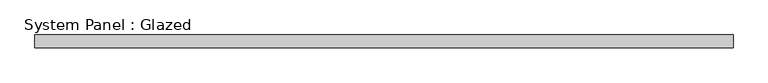
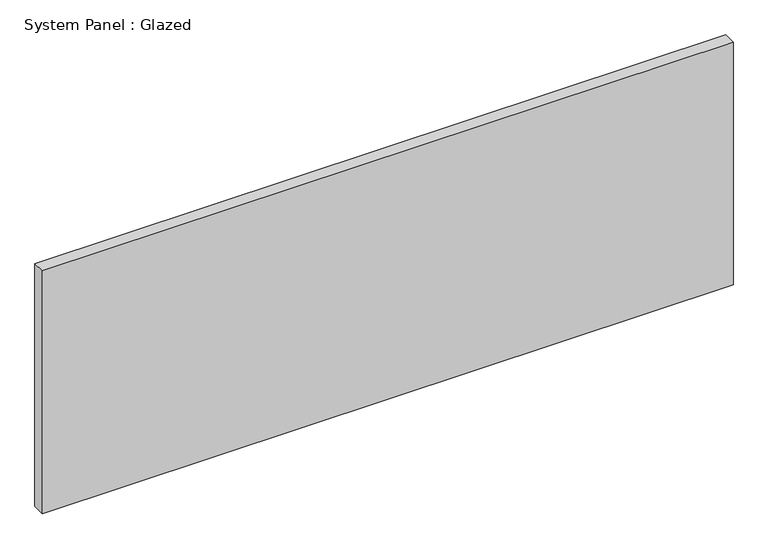
"""IFC4 building model written with IfcOpenShell, lengths in millimetres: plate geometry, System Panel : Glazed."""

from ifc_helpers import new_model, si_unit, origin, origin_with_axes, place, context, project, spatial, polyline, outline, extrude, source, transform, mapped, element, save


def system_panel_glazed_94232cd9(model_context):
    return source(origin(), model_context, "Body", "SweptSolid", [
        extrude(outline(polyline([(692.15, 19.05), (-692.15, 19.05), (-692.15, 44.45), (692.15, 44.45), (692.15, 19.05)])), origin_with_axes(), (0.0, 0.0, 1.0), 514.35),
    ])


if __name__ == "__main__":
    model = new_model("IFC4")
    model_context = context("Model", 3, world=origin())
    ifc_project = project(units=[si_unit("LENGTHUNIT", "METRE", prefix="MILLI")], contexts=[model_context])
    site = spatial("IfcSite", under=ifc_project)
    building = spatial("IfcBuilding", under=site)
    placement = place(None, origin())
    system_panel_glazed_shape = system_panel_glazed_94232cd9(model_context)
    element("IfcPlate", 1, ObjectType="System Panel : Glazed", at=placement, inside=building, context=model_context, shape_type="MappedRepresentation", body=[
        mapped(system_panel_glazed_shape, transform((0.0, 0.0, 0.0), x_axis=(1.0, 0.0, 0.0), y_axis=(0.0, 1.0, 0.0), z_axis=(0.0, 0.0, 1.0))),
    ])
    save(model, "model.ifc")

# Revit data of these elements
# Type "System Panel : Glazed"
#   Construction Type Id = "GSP4R"
#   Analytic Construction = "1/8 in Pilkington single glazing"
#   Visual Light Transmittance = 0.9
#   Solar Heat Gain Coefficient = 0.86
#   Heat Transfer Coefficient (U) = 1.18115 BTU/(h·ft²·°F)
# Element 1 (IfcPlate, "System Panel : Glazed")
#   Materials on its faces: "Glass"
# Materials
#   "Glass": class "Glass", colour RGB 0 128 192, transparency 0.75, Description = "Soda Lime Glass", Cost = 0
